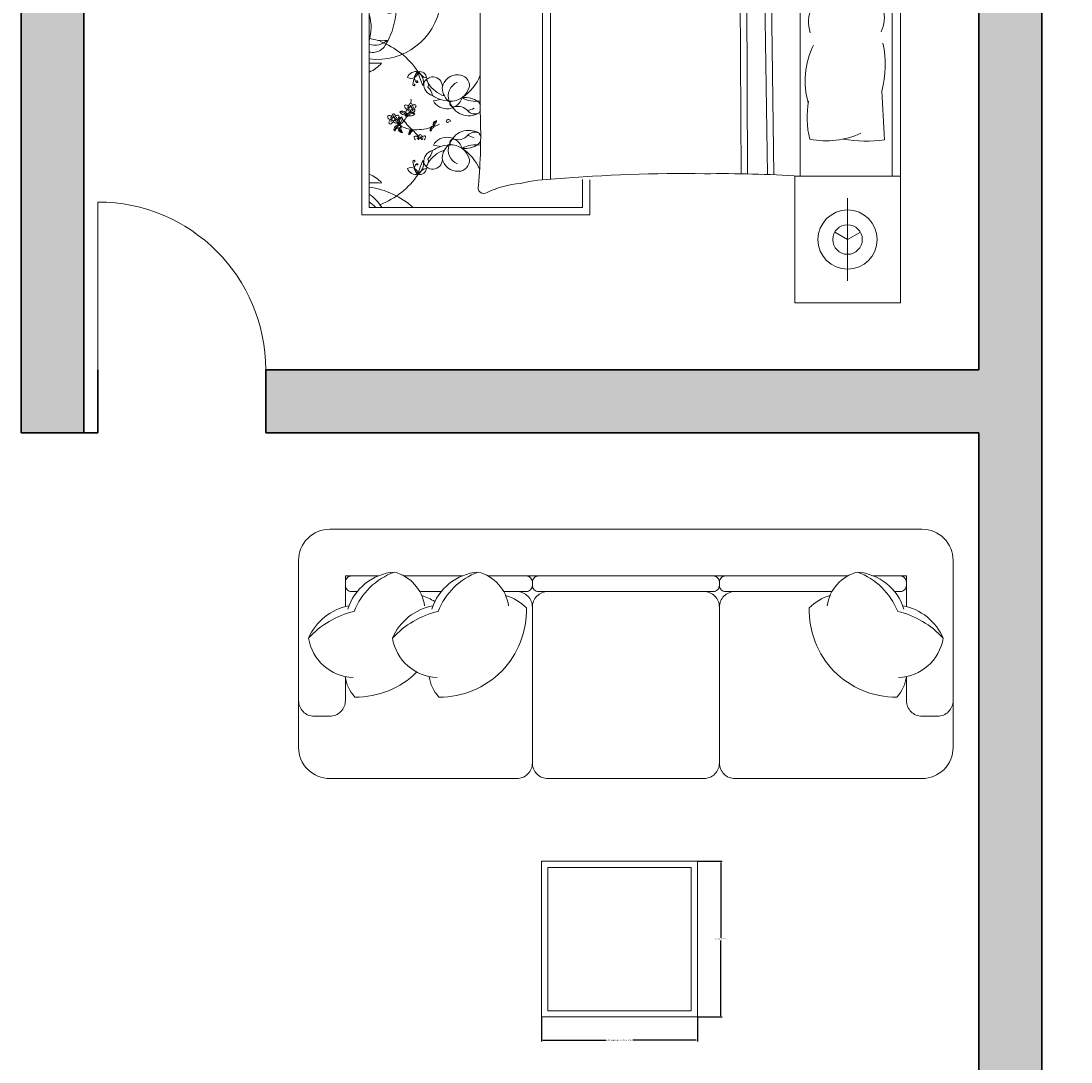
# Model space of a CAD drawing. Units: inches. Extents: x 37 to 706, y -568 to 110.
# Tile 19 of 24: x 212 to 362, y -233 to -84. Entities that reach past the tile are written whole.
import ezdxf

# ---------------------------------------------------------------- set-up
doc = ezdxf.new("R2010")
doc.units = ezdxf.units.IN
doc.header["$MEASUREMENT"] = 0
for name, color, linetype, lineweight in [('A-ANNO-DIMS', 2, 'Continuous', 18), ('A-DOOR', 4, 'Continuous', 18), ('A-FURN', 8, 'Continuous', 13), ('A-WALL', 7, 'Continuous', 35), ('A-WALL-PATT', 252, 'Continuous', 13)]:
    doc.layers.add(name, color=color, linetype=linetype, lineweight=lineweight)
doc.styles.get("Standard").update_dxf_attribs({"font": 'arial.ttf'})
doc.dimstyles.get("Standard").update_dxf_attribs({"dimtxt": 0.18, "dimasz": 0.18, "dimexe": 0.18, "dimexo": 0.0625, "dimgap": 0.09, "dimtad": 0, "dimtih": 1, "dimtoh": 1, "dimdec": 0, "dimzin": 0, "dimdsep": 46, "dimlunit": 3, "dimtxsty": 'Standard', "dimcen": 0.09, "dimadec": 0, "dimazin": 0, "dimtfac": 1, "dimtdec": 0, "dimtofl": 0, "dimtmove": 0, "dimatfit": 3, "dimfxl": 1, "dimtolj": 1, "dimtzin": 0, "dimarcsym": 0})

# ---------------------------------------------------------------- blocks, each defined once
blk = doc.blocks.new('BED-DOUBLE-WITH-NIGHTSTANDS')
for p, q in [((77.02, 90.57), (77.02, 0)), ((69.47, 75.59), (69.47, 87.43)), ((63.56, 81.51), (75.39, 81.51)), ((0, 78.61), (32.62, 78.61)), ((0, 12.59), (0, 78.61)), ((32.62, 78.61), (32.62, 73.49)), ((1.05, 77.56), (1.05, 13.64)), ((31.58, 77.56), (1.05, 77.56)), ((31.58, 73.49), (31.58, 77.56)), ((25.85, 17.62), (25.85, 73.5)), ((26.98, 17.7), (26.98, 73.5)), ((50.48, 72.53), (51.22, 73.26)), ((50.85, 68.86), (50.48, 72.53)), ((51.22, 73.26), (55.07, 69.96)), ((77.02, 72.45), (52.16, 72.45)), ((62.71, 72.45), (62.71, 18.11)), ((75.86, 18.11), (75.86, 72.45)), ((55.07, 69.96), (57.63, 66.48)), ((10.23, 68.64), (11.25, 68.84)), ((50.48, 64.28), (50.85, 68.86)), ((57.63, 66.48), (60.02, 59.87)), ((16.95, 26.9), (16.95, 63.67)), ((49.93, 60.24), (50.48, 64.28)), ((10.23, 62.31), (11.25, 62.11)), ((48.83, 57.86), (49.93, 60.24)), ((60.02, 59.87), (62.71, 50)), ((48.1, 54.92), (48.83, 57.86)), ((50.48, 54.55), (48.1, 54.92)), ((55.8, 52.54), (50.48, 54.55)), ((54.24, 18.43), (54.09, 53.18)), ((55.17, 18.44), (55.03, 52.83)), ((62.71, 47.57), (55.8, 52.54)), ((58.02, 18.39), (57.55, 51.28)), ((58.95, 18.36), (58.49, 50.6)), ((10.23, 28.89), (11.25, 29.09)), ((10.23, 22.56), (11.25, 22.36)), ((31.58, 13.64), (31.58, 17.63)), ((32.62, 17.61), (32.62, 12.59)), ((1.05, 13.64), (31.58, 13.64)), ((69.47, 14.97), (69.47, 3.14)), ((32.62, 12.59), (0, 12.59))]:
    blk.add_line(p, q)
for points in [[(61.93, 72.45), (61.93, 90.57), (77.02, 90.57)], [(69.47, 81.51), (67.64, 80.45)], [(69.47, 81.51), (71.3, 80.45)], [(77.02, 18.11), (61.93, 18.11), (61.93, 0), (77.02, 0)], [(69.47, 9.06), (67.64, 10.11)], [(69.47, 9.06), (71.3, 10.11)]]:
    blk.add_lwpolyline(points)
for points in [[(42.92, 73.45, 0.001242), (25.74, 73.5, -0.127202), (17.18, 75.31)], [(74.76, 67.25, 0.074897), (68.85, 67.14, -0.472817)], [(68.52, 45.71, 0.14099), (74.55, 45.53, 0.235245)], [(68.52, 41.84, -0.14099), (74.55, 42.02, -0.235245)], [(74.76, 23.32, -0.074897), (68.85, 23.42, 0.472817)], [(27.69, 17.73, 0.056112), (22.71, 17.07, 0.095341), (17.91, 15.8)]]:
    blk.add_lwpolyline(points, format="xyb")
for centre, radius in [((69.47, 81.51), 4.23), ((69.47, 81.51), 2.11), ((4.52, 64.91), 0.231), ((6.95, 63.41), 0.231), ((6.95, 27.79), 0.231), ((4.52, 26.28), 0.231), ((69.47, 9.06), 4.23), ((69.47, 9.06), 2.11)]:
    blk.add_circle(centre, radius)
for centre, radius, start, end in [((-3.2, 82.51), 7.18, 306.3036, 316.4814), ((-2.13, 80.43), 5.76, 303.4617, 330.1116), ((-0.54, 86.37), 11.83, 277.745, 311.8856), ((-1.71, 66.13), 11.83, 34.3865, 68.5908), ((17.23, 74.48), 0.836, 93.98, 207.3412), ((-0.79, 77.21), 4.81, 292.5547, 318.9546), ((1.79, 90.38), 16.36, 267.4081, 273.6519), ((-77.32, 64.75), 94.28, 359.3433, 5.6887), ((7.77, 71.53), 1.31, 77.7115, 159.0387), ((7.06, 72.84), 0.988, 238.4633, 358.2869), ((10.3, 70.85), 2.99, 138.8402, 177.9352), ((8.5, 71.96), 0.967, 117.6827, 223.7762), ((8.28, 71.86), 0.98, 2.9516, 103.728), ((16.12, 74.61), 8.27, 192.5173, 207.1824), ((6.95, 71.3), 1.87, 345.4653, 54.2343), ((9.77, 73.87), 2.02, 211.3827, 255.2969), ((13.65, 70.21), 2.16, 84.9449, 172.8857), ((13.86, 70.84), 1.53, 354.4856, 91.0538), ((48.97, 156.3), 83.07, 265.8294, 271.553), ((83.29, 71.71), 34.18, 177.4519, 191.3392), ((7.46, 70.95), 0.147, 177.9352, 11.4834), ((7.53, 70.96), 0.0713, 11.4834, 127.9409), ((7.89, 71.38), 0.128, 223.7762, 159.7183), ((10.16, 70.71), 1.36, 350.264, 160.8688), ((10.57, 71.04), 1.7, 175.969, 254.3045), ((8.69, 70.99), 0.833, 333.9755, 53.2681), ((8.31, 69.21), 1.81, 6.1662, 51.5825), ((13.15, 73.4), 4.28, 211.2614, 251.7045), ((14.47, 69.36), 2.1, 111.5819, 201.4221), ((12.73, 71.31), 2.72, 265.2933, 346.921), ((10.57, 74.83), 6.85, 303.6671, 333.2997), ((12.81, 73.44), 4.86, 236.2883, 266.5076), ((12.18, 69.76), 2.25, 209.9085, 343.1337), ((14.13, 70.59), 2.63, 182.3591, 234.0401), ((16.28, 72.32), 3.75, 238.8218, 279.1554), ((14.65, 65.65), 3.49, 55.785, 94.7304), ((7.66, 67.53), 0.177, 142.4737, 265.053), ((7.89, 67.56), 0.381, 127.7621, 169.0403), ((7.69, 67.89), 0.536, 265.053, 338.3618), ((8.4, 67.15), 0.7, 113.4276, 137.6104), ((8.32, 67.88), 0.231, 183.2768, 356.7232), ((8.49, 67.46), 0.377, 139.7889, 227.6792), ((7.6, 67.46), 0.755, 353.0852, 15.7171), ((8.1, 67.37), 0.477, 350.3487, 43.6538), ((8.98, 67.87), 0.555, 198.7263, 262.5032), ((8.54, 67.61), 0.22, 1.1081, 91.8675), ((8.68, 67.56), 0.385, 11.5637, 52.6358), ((8.95, 67.49), 0.178, 255.2356, 54.9248), ((13.13, 68.34), 0.562, 167.3041, 285.1471), ((14.65, 65.65), 3.49, 122.7011, 126.3445), ((15.31, 69.41), 2.89, 199.2822, 299.1751), ((13.76, 66), 1.86, 41.5653, 105.1471), ((14.78, 69.85), 2.6, 277.436, 299.9149), ((15.95, 67.67), 1.09, 30.0293, 52.325), ((4.85, 66.4), 0.258, 124.3538, 214.3923), ((5.23, 66.36), 0.6, 190.3057, 287.1958), ((5.41, 66.58), 0.697, 176.9701, 248.2913), ((10.38, 70.25), 6.74, 212.6784, 216.3746), ((5.17, 66.41), 0.267, 216.3746, 291.7548), ((5.81, 66.23), 0.6, 122.8155, 187.3992), ((5.34, 65.98), 0.201, 289.3605, 111.7548), ((5.49, 65.98), 0.201, 221.8703, 44.2646), ((6.07, 66.15), 0.697, 109.4799, 177.6828), ((5.7, 66.59), 0.258, 56.8636, 146.9021), ((5.83, 66.31), 0.267, 148.8844, 224.2646), ((11.37, 62.96), 6.74, 145.1882, 148.8844), ((7.53, 62.67), 3.76, 94.756, 119.2041), ((15.54, 57.26), 12.37, 132.2412, 142.1744), ((9.29, 67.11), 2.55, 178.3264, 187.1302), ((6.53, 66.75), 0.476, 11.3256, 64.4621), ((8.15, 67.44), 1.43, 190.2588, 210.656), ((7.19, 66.85), 0.435, 188.3432, 274.2869), ((7.57, 67.09), 0.759, 210.656, 242.6341), ((8.14, 67.75), 1.46, 218.2101, 226.3071), ((7.07, 66.52), 0.185, 325.7657, 67.4417), ((1.34, 72.69), 8.6, 313.1541, 322.0459), ((7.72, 58.94), 7.5, 73.5842, 93.8277), ((8.37, 67.33), 0.199, 227.6792, 350.3487), ((12.34, 66.57), 2.55, 178.3264, 187.1302), ((9.58, 66.21), 0.476, 11.3256, 64.4621), ((11.19, 66.9), 1.43, 190.2588, 210.656), ((10.23, 66.31), 0.435, 188.3432, 274.2869), ((10.61, 66.55), 0.759, 210.656, 242.6341), ((11.19, 67.21), 1.46, 218.2101, 226.3071), ((10.11, 65.98), 0.185, 325.7657, 67.4417), ((16.16, 68.13), 1.36, 221.5653, 293.8354), ((15.95, 67.67), 1.09, 314.4517, 333.558), ((75.82, 64.02), 12.14, 165.1039, 191.0369), ((66.47, 55.71), 11.67, 65.1316, 101.7583), ((936.66, 17.33), 863.34, 176.68521, 177.14978), ((3.86, 64.56), 0.177, 142.4737, 265.053), ((4.09, 64.6), 0.381, 61.2196, 169.0403), ((3.89, 64.92), 0.536, 265.053, 338.3618), ((4.34, 65.38), 0.455, 157.4086, 261.4386), ((4.09, 65.4), 0.229, 58.0499, 135.6268), ((4.6, 64.19), 0.7, 113.4276, 137.6104), ((4.32, 65.26), 0.153, 172.906, 277.132), ((3.82, 64.98), 0.727, 14.7558, 58.0499), ((4.69, 64.5), 0.377, 139.7889, 227.6792), ((4.84, 65.17), 0.315, 36.1046, 181.4281), ((3.8, 64.5), 0.755, 353.0852, 15.7171), ((4.29, 64.41), 0.477, 350.3487, 43.6538), ((5.18, 64.9), 0.555, 198.7263, 262.5032), ((4.66, 65.42), 0.317, 270.0645, 331.1507), ((4.93, 65.34), 0.363, 221.8413, 265.7877), ((4.74, 64.65), 0.22, 1.1081, 91.8675), ((4.92, 65.2), 0.226, 263.7526, 41.7054), ((4.88, 64.6), 0.385, 11.5637, 86.365), ((7.53, 62.67), 3.76, 124.0033, 132.4917), ((5.15, 64.53), 0.178, 255.2356, 54.9248), ((3.66, 62.2), 4.02, 63.7819, 68.2913), ((5.81, 65.29), 0.639, 128.3208, 208.8162), ((5.92, 65.34), 0.764, 207.7043, 254.3516), ((6.41, 65.39), 1.05, 157.2305, 229.0635), ((6.05, 65.74), 0.619, 174.4544, 220.6188), ((5.43, 64.9), 1.05, 270.278, 342.111), ((2.53, 62.29), 4.51, 30.544, 49.818), ((5.02, 64.86), 0.744, 340.0041, 40.6188), ((5.92, 64.93), 0.619, 278.7227, 324.8872), ((7.06, 64.61), 0.639, 182.8499, 266.1226), ((6.81, 65.06), 0.619, 231.7607, 277.9252), ((7.29, 65.17), 1.05, 214.5369, 286.3699), ((10.63, 65.65), 0.435, 147.5332, 233.4768), ((11.02, 65.87), 0.759, 179.1859, 211.164), ((10.28, 65.7), 0.185, 354.3784, 96.0543), ((7.72, 58.94), 7.5, 63.0032, 69.8941), ((11.6, 66.22), 1.43, 211.164, 231.5612), ((11.85, 67.38), 2.55, 234.6898, 243.4936), ((11.87, 66.07), 1.46, 195.5129, 203.6099), ((10.23, 65.12), 0.476, 357.3579, 50.4944), ((12.28, 65.21), 0.175, 12.7051, 190.4384), ((12.38, 65.23), 0.284, 190.4384, 10.4136), ((42.55, 63.54), 7.37, 336.2616, 11.3392), ((4.57, 64.37), 0.199, 227.6792, 350.3487), ((6.13, 63.58), 0.744, 98.7227, 159.3375), ((5.75, 64.54), 0.764, 244.9899, 291.6373), ((5.81, 64.43), 0.639, 290.5253, 358.5375), ((6.29, 63.06), 0.177, 142.4737, 265.053), ((6.52, 63.09), 0.381, 61.2196, 169.0403), ((6.32, 63.41), 0.536, 265.053, 338.3618), ((6.77, 63.88), 0.455, 157.4086, 261.4386), ((6.52, 63.89), 0.229, 58.0499, 135.6268), ((7.03, 62.68), 0.7, 113.4276, 137.6104), ((6.76, 63.75), 0.153, 172.906, 277.132), ((6.25, 63.47), 0.727, 14.7558, 58.0499), ((2.53, 62.29), 4.51, 23.0501, 23.8477), ((7.12, 62.99), 0.377, 139.7889, 227.6792), ((7, 63.71), 0.744, 37.3105, 97.9252), ((7.27, 63.66), 0.315, 36.1046, 181.4281), ((6.23, 62.99), 0.755, 353.0852, 15.7171), ((7.08, 64.73), 0.764, 265.0106, 311.658), ((6.72, 62.9), 0.477, 350.3487, 43.6538), ((7.61, 63.4), 0.555, 198.7263, 262.5032), ((7.09, 63.91), 0.317, 270.0645, 331.1507), ((7.36, 63.83), 0.363, 221.8413, 265.7877), ((7.17, 63.14), 0.22, 1.1081, 91.8675), ((7.36, 63.7), 0.226, 263.7526, 41.7054), ((7.31, 63.09), 0.385, 11.5637, 86.365), ((7.58, 63.02), 0.178, 255.2356, 54.9248), ((12.18, 61.19), 2.25, 16.8663, 150.0915), ((13.13, 62.61), 0.562, 74.8529, 192.6959), ((15.31, 61.54), 2.89, 60.8249, 160.7178), ((13.76, 64.95), 1.86, 254.8529, 318.4347), ((14.78, 61.1), 2.6, 60.0851, 82.564), ((16.16, 62.82), 1.36, 66.1646, 138.4347), ((15.95, 63.28), 1.09, 23.229, 45.5483), ((7, 62.86), 0.199, 227.6792, 350.3487), ((2.53, 62.29), 4.51, 357.1071, 4.7585), ((13.15, 57.54), 4.28, 108.2955, 148.7386), ((12.81, 57.5), 4.86, 93.4924, 123.7117), ((14.13, 60.36), 2.63, 125.9599, 177.6409), ((14.47, 61.59), 2.1, 158.5779, 248.4181), ((12.73, 59.64), 2.72, 13.079, 94.7067), ((14.65, 65.3), 3.49, 233.6555, 237.2989), ((16.28, 58.63), 3.75, 79.7133, 121.1782), ((14.65, 65.3), 3.49, 265.2696, 304.215), ((10.57, 56.11), 6.85, 21.4941, 56.3329), ((15.95, 63.28), 1.09, 307.675, 336.7144), ((84.45, 57.63), 21.05, 168.0397, 199.2615), ((7.46, 60), 0.147, 348.5166, 182.0648), ((6.95, 59.65), 1.87, 305.7657, 14.5347), ((16.12, 56.34), 8.27, 152.8176, 167.4827), ((10.57, 59.91), 1.7, 105.6955, 184.031), ((10.16, 60.24), 1.36, 199.1312, 9.736), ((8.69, 59.96), 0.833, 306.7319, 26.0245), ((8.31, 61.74), 1.81, 308.4175, 353.8338), ((13.65, 60.74), 2.16, 187.1143, 275.0551), ((13.86, 60.11), 1.53, 268.9462, 5.5144), ((82.33, 48.63), 35.12, 160.1194, 169.3383), ((41.99, 54.84), 32.85, 352.2196, 9.497), ((7.06, 58.1), 0.988, 1.7131, 121.5367), ((7.77, 59.41), 1.31, 200.9613, 282.2885), ((10.3, 60.1), 2.99, 182.0648, 221.1598), ((7.53, 59.98), 0.0713, 232.0591, 348.5166), ((8.5, 58.99), 0.967, 136.2238, 242.3173), ((7.94, 59.56), 0.0771, 200.2667, 136.2271), ((8.28, 59.09), 0.98, 256.272, 357.0484), ((9.77, 57.08), 2.02, 104.7031, 148.6173), ((-0.79, 53.74), 4.81, 41.0454, 67.4453), ((-1.71, 64.81), 11.83, 291.4092, 325.6135), ((1.79, 40.57), 16.36, 86.3481, 92.5919), ((-0.54, 44.58), 11.83, 4.4623, 82.255), ((-2.13, 50.51), 5.76, 1.272, 56.5383), ((-3.2, 48.44), 7.18, 17.8504, 53.6964), ((48.03, 55.13), 0.219, 178.8623, 289.7536), ((-5.22, 44.66), 10.68, 34.0123, 54.053), ((79.85, 49.11), 15.97, 169.8617, 193.6238), ((58.59, 47.9), 16.14, 351.5249, 13.96), ((-5.17, 48.79), 6.5, 343.5431, 17.0202), ((-6.88, 45.48), 11.83, 4.4623, 27.4146), ((-8.52, 46.22), 9.62, 4.3787, 5.6357), ((-15.11, 41.15), 17.18, 19.7217, 19.9028), ((4.03, 45.43), 1.31, 47.7873, 129.1145), ((4.07, 46.92), 0.988, 208.5391, 328.3627), ((3.47, 45.08), 0.147, 148.011, 341.5592), ((5.88, 43.58), 2.99, 108.9159, 148.011), ((3.54, 45.06), 0.0713, 341.5592, 98.0167), ((4.87, 45.44), 0.967, 87.7585, 193.852), ((4.06, 45.24), 0.128, 193.852, 129.9245), ((12.81, 43.93), 8.27, 162.593, 177.2582), ((3.21, 45.64), 1.87, 315.5411, 24.3101), ((6.93, 46.46), 2.02, 181.4585, 225.3727), ((4.64, 45.46), 0.98, 333.0274, 73.8037), ((10.37, 44.53), 1.31, 47.7873, 129.1145), ((10.41, 46.02), 0.988, 208.5391, 328.3627), ((12.22, 42.67), 2.99, 108.9159, 148.011), ((11.21, 44.53), 0.967, 87.7585, 193.852), ((9.54, 44.73), 1.87, 315.5411, 24.3101), ((19.14, 43.02), 8.27, 162.593, 177.2582), ((10.97, 44.56), 0.98, 333.0274, 73.8037), ((13.27, 45.55), 2.02, 181.4585, 225.3727), ((65.49, 56.38), 11.1, 264.0129, 285.8293), ((12.81, 44.25), 8.27, 182.7418, 197.407), ((3.21, 42.54), 1.87, 335.6899, 44.4589), ((9.8, 44.18), 0.147, 148.011, 341.5592), ((9.8, 44), 0.147, 18.4408, 211.989), ((12.22, 45.51), 2.99, 211.989, 251.0841), ((9.88, 44.15), 0.0713, 341.5592, 98.0167), ((9.88, 44.03), 0.0713, 261.9833, 18.4408), ((11.21, 43.65), 0.967, 166.148, 272.2415), ((10.39, 44.33), 0.128, 193.852, 129.9245), ((10.44, 43.86), 0.0771, 230.1909, 166.0209), ((9.54, 43.45), 1.87, 335.6899, 44.4589), ((19.14, 45.16), 8.27, 182.7418, 197.407), ((10.97, 43.62), 0.98, 286.1963, 26.9726), ((13.27, 42.63), 2.02, 134.6273, 178.5415), ((2.19, 43.98), 9.15, 262.8636, 351.8197), ((4.07, 41.26), 0.988, 31.6373, 151.4609), ((3.47, 43.1), 0.147, 18.4408, 211.989), ((5.88, 44.6), 2.99, 211.989, 251.0841), ((3.54, 43.12), 0.0713, 261.9833, 18.4408), ((4.87, 42.74), 0.967, 166.148, 272.2415), ((4.11, 42.95), 0.0771, 230.1909, 166.0209), ((6.93, 41.72), 2.02, 134.6273, 178.5415), ((4.64, 42.72), 0.98, 286.1963, 26.9726), ((10.41, 42.16), 0.988, 31.6373, 151.4609), ((10.37, 43.65), 1.31, 230.8855, 312.2127), ((68.68, 40.17), 4.8, 155.0183, 198.5407), ((65.49, 31.16), 11.1, 74.1707, 95.9871), ((-5.17, 39.39), 6.5, 342.9798, 16.4569), ((-8.52, 41.96), 9.62, 354.3643, 355.6213), ((-15.11, 47.03), 17.18, 340.0972, 340.2783), ((4.03, 42.75), 1.31, 230.8855, 312.2127), ((-6.88, 42.69), 11.83, 332.5854, 355.5377), ((70.25, 40.78), 4.48, 333.3437, 16.1026), ((3.02, 42.8), 5.3, 248.117, 276.6195), ((1.55, 37.94), 2.12, 256.3898, 349.0739), ((1.84, 39.54), 2.68, 252.8609, 311.9049), ((-1.71, 26.39), 11.83, 34.3865, 68.5908), ((74.93, 31.78), 11.53, 153.8761, 196.1746), ((58.92, 34.06), 15.92, 346.3427, 11.1841), ((1.79, 50.63), 16.36, 267.4081, 273.6519), ((-0.79, 37.46), 4.81, 292.5547, 318.9546), ((7.77, 31.78), 1.31, 77.7115, 159.0387), ((7.06, 33.09), 0.988, 238.4633, 358.2869), ((10.3, 31.1), 2.99, 138.8402, 177.9352), ((8.5, 32.21), 0.967, 117.6827, 223.7762), ((8.28, 32.11), 0.98, 2.9516, 103.728), ((9.77, 34.12), 2.02, 211.3827, 255.2969), ((6.95, 31.55), 1.87, 345.4653, 54.2343), ((16.12, 34.86), 8.27, 192.5173, 207.1824), ((7.89, 31.63), 0.128, 223.7762, 159.7183), ((10.16, 30.96), 1.36, 350.264, 160.8688), ((8.69, 31.24), 0.833, 333.9755, 53.2681), ((13.65, 30.46), 2.16, 84.9449, 172.8857), ((14.47, 29.61), 2.1, 111.5819, 201.4221), ((13.86, 31.09), 1.53, 354.4856, 91.0538), ((10.57, 35.08), 6.85, 303.6671, 338.5059), ((7.46, 31.2), 0.147, 177.9352, 11.4834), ((7.53, 31.21), 0.0713, 11.4834, 127.9409), ((10.57, 31.29), 1.7, 175.969, 254.3045), ((8.31, 29.46), 1.81, 6.1662, 51.5825), ((13.15, 33.66), 4.28, 211.2614, 251.7045), ((14.13, 30.84), 2.63, 182.3591, 234.0401), ((12.73, 31.56), 2.72, 265.2933, 346.921), ((936.66, 73.23), 863.34, 182.85022, 183.31479), ((7, 28.34), 0.199, 9.6513, 132.3208), ((2.53, 28.91), 4.51, 355.2415, 2.8929), ((12.81, 33.7), 4.86, 236.2883, 266.5076), ((12.18, 30.01), 2.25, 209.9085, 343.1337), ((13.13, 28.59), 0.562, 167.3041, 285.1471), ((14.65, 25.9), 3.49, 122.7011, 126.3445), ((15.31, 29.66), 2.89, 199.2822, 299.1751), ((16.28, 32.57), 3.75, 238.8218, 280.2867), ((14.65, 25.9), 3.49, 55.785, 94.7304), ((15.95, 27.92), 1.09, 23.2856, 52.325), ((75.82, 26.55), 12.14, 168.9631, 194.8961), ((4.57, 26.83), 0.199, 9.6513, 132.3208), ((5.75, 26.66), 0.764, 68.3627, 115.0101), ((5.43, 26.3), 1.05, 17.889, 89.722), ((6.13, 27.61), 0.744, 200.6625, 261.2773), ((5.81, 26.77), 0.639, 1.4625, 69.4747), ((6.29, 28.14), 0.177, 94.947, 217.5263), ((6.52, 28.11), 0.381, 190.9597, 298.7804), ((6.32, 27.78), 0.536, 21.6382, 94.947), ((6.77, 27.32), 0.455, 98.5614, 202.5914), ((6.52, 27.31), 0.229, 224.3732, 301.9501), ((7.06, 26.59), 0.639, 93.8774, 177.1501), ((7.29, 26.03), 1.05, 73.6301, 145.4631), ((7.03, 28.52), 0.7, 222.3896, 246.5724), ((6.76, 27.45), 0.153, 82.868, 187.094), ((6.25, 27.73), 0.727, 301.9501, 345.2442), ((2.53, 28.91), 4.51, 336.1523, 336.9499), ((7.12, 28.21), 0.377, 132.3208, 220.2111), ((7, 27.49), 0.744, 262.0748, 322.6895), ((6.23, 28.2), 0.755, 344.2829, 6.9148), ((7.27, 27.54), 0.315, 178.5719, 323.8954), ((7.08, 26.46), 0.764, 48.342, 94.9894), ((6.72, 28.3), 0.477, 316.3462, 9.6513), ((7.61, 27.8), 0.555, 97.4968, 161.2737), ((7.36, 27.37), 0.363, 94.2123, 138.1587), ((7.09, 27.29), 0.317, 28.8493, 89.9355), ((7.17, 28.06), 0.22, 268.1325, 358.8919), ((7.31, 28.11), 0.385, 273.635, 348.4363), ((7.36, 27.5), 0.226, 318.2946, 96.2474), ((7.58, 28.18), 0.178, 305.0752, 104.7644), ((13.76, 26.25), 1.86, 41.5653, 105.1471), ((14.78, 30.1), 2.6, 277.436, 299.9149), ((16.16, 28.38), 1.36, 221.5653, 293.8354), ((15.95, 27.92), 1.09, 314.4517, 336.7144), ((3.86, 26.63), 0.177, 94.947, 217.5263), ((4.09, 26.6), 0.381, 190.9597, 298.7804), ((3.89, 26.28), 0.536, 21.6382, 94.947), ((4.34, 25.81), 0.455, 98.5614, 202.5914), ((4.09, 25.8), 0.229, 224.3732, 301.9501), ((4.6, 27.01), 0.7, 222.3896, 246.5724), ((4.32, 25.94), 0.153, 82.868, 187.094), ((3.82, 26.22), 0.727, 301.9501, 345.2442), ((4.69, 26.7), 0.377, 132.3208, 220.2111), ((4.84, 26.03), 0.315, 178.5719, 323.8954), ((3.8, 26.7), 0.755, 344.2829, 6.9148), ((4.29, 26.79), 0.477, 316.3462, 9.6513), ((5.18, 26.29), 0.555, 97.4968, 161.2737), ((4.93, 25.86), 0.363, 94.2123, 138.1587), ((4.66, 25.78), 0.317, 28.8493, 89.9355), ((4.74, 26.55), 0.22, 268.1325, 358.8919), ((4.88, 26.6), 0.385, 273.635, 348.4363), ((4.92, 25.99), 0.226, 318.2946, 96.2474), ((7.53, 28.53), 3.76, 227.5083, 235.9967), ((5.15, 26.67), 0.178, 305.0752, 104.7644), ((5.81, 25.91), 0.639, 151.1838, 231.6792), ((5.92, 25.86), 0.764, 105.6484, 152.2957), ((6.41, 25.8), 1.05, 130.9365, 202.7695), ((6.05, 25.46), 0.619, 139.3812, 185.5456), ((2.53, 28.91), 4.51, 310.182, 329.456), ((5.02, 26.34), 0.744, 319.3812, 19.9959), ((15.54, 33.94), 12.37, 217.8256, 227.7588), ((5.92, 26.27), 0.619, 35.1128, 81.2773), ((6.81, 26.14), 0.619, 82.0748, 128.2393), ((10.63, 25.55), 0.435, 126.5232, 212.4668), ((11.02, 25.33), 0.759, 148.836, 180.8141), ((7.72, 32.26), 7.5, 290.1059, 296.9968), ((11.6, 24.98), 1.43, 128.4388, 148.836), ((11.85, 23.82), 2.55, 116.5064, 125.3102), ((11.87, 25.13), 1.46, 156.3901, 164.4871), ((10.23, 26.08), 0.476, 309.5056, 2.6421), ((12.28, 25.98), 0.175, 169.5616, 347.2949), ((12.38, 25.96), 0.284, 349.5864, 169.5616), ((-71.13, 24.12), 88.13, 355.2402, 1.8035), ((4.85, 24.8), 0.258, 145.6077, 235.6462), ((5.23, 24.83), 0.6, 72.8042, 169.6943), ((5.41, 24.62), 0.697, 111.7087, 183.0299), ((10.38, 20.95), 6.74, 143.6254, 147.3216), ((5.17, 24.78), 0.267, 68.2452, 143.6254), ((3.66, 29), 4.02, 291.7087, 296.2181), ((5.81, 24.97), 0.6, 172.6008, 237.1845), ((5.34, 25.22), 0.201, 248.2452, 70.6395), ((5.49, 25.22), 0.201, 315.7354, 138.1297), ((6.07, 25.05), 0.697, 182.3172, 250.5201), ((5.7, 24.61), 0.258, 213.0979, 303.1364), ((5.83, 24.89), 0.267, 135.7354, 211.1156), ((11.37, 28.24), 6.74, 211.1156, 214.8118), ((7.53, 28.53), 3.76, 240.7959, 265.244), ((8.15, 23.76), 1.43, 149.344, 169.7412), ((9.29, 24.09), 2.55, 172.8698, 181.6736), ((6.53, 24.45), 0.476, 295.5379, 348.6744), ((7.19, 24.34), 0.435, 85.7131, 171.6568), ((7.57, 24.1), 0.759, 117.3659, 149.344), ((8.14, 23.45), 1.46, 133.6929, 141.7899), ((7.07, 24.67), 0.185, 292.5583, 34.2343), ((7.72, 32.26), 7.5, 266.1723, 286.4158), ((1.34, 18.5), 8.6, 37.9541, 46.8459), ((8.37, 23.87), 0.199, 9.6513, 132.3208), ((11.19, 24.3), 1.43, 149.344, 169.7412), ((12.34, 24.63), 2.55, 172.8698, 181.6736), ((9.58, 24.98), 0.476, 295.5379, 348.6744), ((10.23, 24.88), 0.435, 85.7131, 171.6568), ((10.61, 24.64), 0.759, 117.3659, 149.344), ((11.19, 23.99), 1.46, 133.6929, 141.7899), ((10.11, 25.21), 0.185, 292.5583, 34.2343), ((10.28, 25.5), 0.185, 263.9457, 5.6216), ((15.31, 21.79), 2.89, 60.8249, 160.7178), ((16.16, 23.07), 1.36, 66.1646, 138.4347), ((15.95, 23.53), 1.09, 16.6343, 45.5483), ((66.47, 34.85), 11.67, 258.2417, 294.8684), ((7.66, 23.67), 0.177, 94.947, 217.5263), ((7.89, 23.64), 0.381, 190.9597, 232.2379), ((7.69, 23.31), 0.536, 21.6382, 94.947), ((8.4, 24.05), 0.7, 222.3896, 246.5724), ((8.32, 23.32), 0.231, 3.2768, 176.7232), ((8.49, 23.74), 0.377, 132.3208, 220.2111), ((7.6, 23.73), 0.755, 344.2829, 6.9148), ((8.1, 23.82), 0.477, 316.3462, 9.6513), ((8.98, 23.33), 0.555, 97.4968, 161.2737), ((8.54, 23.59), 0.22, 268.1325, 358.8919), ((8.95, 23.71), 0.178, 305.0752, 104.7644), ((8.68, 23.64), 0.385, 307.3642, 348.4363), ((12.81, 17.75), 4.86, 93.4924, 123.7117), ((12.18, 21.44), 2.25, 16.8663, 150.0915), ((14.13, 20.61), 2.63, 125.9599, 177.6409), ((14.47, 21.84), 2.1, 158.5779, 248.4181), ((12.73, 19.89), 2.72, 13.079, 94.7067), ((13.13, 22.86), 0.562, 74.8529, 192.6959), ((14.65, 25.55), 3.49, 233.6555, 237.2989), ((13.76, 25.2), 1.86, 254.8529, 318.4347), ((16.28, 18.88), 3.75, 79.249, 121.1782), ((14.65, 25.55), 3.49, 265.2696, 304.215), ((14.78, 21.35), 2.6, 60.0851, 82.564), ((15.95, 23.53), 1.09, 307.675, 342.5814), ((10.57, 20.16), 1.7, 105.6955, 184.031), ((8.31, 21.99), 1.81, 308.4175, 353.8338), ((13.15, 17.79), 4.28, 108.2955, 148.7386), ((10.57, 16.37), 6.85, 23.6453, 56.3329), ((7.46, 20.25), 0.147, 348.5166, 182.0648), ((10.3, 20.35), 2.99, 182.0648, 221.1598), ((7.53, 20.24), 0.0713, 232.0591, 348.5166), ((8.5, 19.24), 0.967, 136.2238, 242.3173), ((7.94, 19.81), 0.0771, 200.2667, 136.2271), ((16.12, 16.59), 8.27, 152.8176, 167.4827), ((6.95, 19.9), 1.87, 305.7657, 14.5347), ((10.16, 20.49), 1.36, 199.1312, 9.736), ((8.69, 20.21), 0.833, 306.7319, 26.0245), ((13.65, 20.99), 2.16, 187.1143, 275.0551), ((13.86, 20.36), 1.53, 268.9462, 5.5144), ((-0.79, 13.99), 4.81, 41.0454, 67.4453), ((-1.71, 25.06), 11.83, 291.4092, 325.6135), ((7.06, 18.36), 0.988, 1.7131, 121.5367), ((7.77, 19.67), 1.31, 200.9613, 282.2885), ((9.77, 17.33), 2.02, 104.7031, 148.6173), ((8.28, 19.34), 0.98, 256.272, 357.0484), ((45.72, -193.78), 212.28, 89.1145, 94.8735), ((51.64, -144.24), 162.73, 86.1, 90.9282), ((1.79, 0.82), 16.36, 86.3481, 92.5919), ((-0.54, 4.83), 11.83, 48.1144, 82.255), ((17.45, 16.48), 0.826, 156.5219, 303.8264), ((-2.13, 10.76), 5.76, 29.8884, 56.5383), ((-3.2, 8.69), 7.18, 43.5186, 53.6964)]:
    blk.add_arc(centre, radius, start, end)
blk = doc.blocks.new('COFFEE-TABLE-SQUARE')
at = {"ltscale": 0.03}
blk.add_lwpolyline([(22.29, 0), (0, 0), (0, 22.29), (22.29, 22.29)], close=True, dxfattribs=at)
blk.add_lwpolyline([(0.89, 0.89), (21.4, 0.89), (21.4, 21.4), (0.89, 21.4)], close=True)
blk = doc.blocks.new('DOOR-SWING-24')
blk.add_line((0, 0), (0, 24))
blk.add_arc((0, 0), 24, 0, 90)
blk = doc.blocks.new('*D35')
at = {"layer": 'A-ANNO-DIMS', "color": 0, "lineweight": -2, "transparency": 16777216}
for p, q in [((286.42, -226.33), (286.42, -229.79)), ((308.71, -226.33), (308.71, -229.79)), ((286.6, -229.61), (295.67, -229.61)), ((308.53, -229.61), (299.46, -229.61))]:
    blk.add_line(p, q, dxfattribs=at)
at = {"layer": 'A-ANNO-DIMS', "color": 0, "transparency": 16777216}
for points in [[(286.6, -229.58), (286.6, -229.64), (286.42, -229.61)], [(308.53, -229.58), (308.53, -229.64), (308.71, -229.61)]]:
    blk.add_solid(points, dxfattribs=at)
at = {"layer": 'Defpoints', "color": 0, "transparency": 16777216}
for p in [(286.42, -226.27), (308.71, -226.27), (308.71, -229.61)]:
    blk.add_point(p, dxfattribs=at)
at = {"layer": 'A-ANNO-DIMS', "color": 0, "transparency": 16777216, "insert": (297.56, -229.61), "char_height": 0.18, "attachment_point": 5}
blk.add_mtext('\\A1;COFFEE TABLE 1\'-10 1/2" TYP.', dxfattribs=at)
blk = doc.blocks.new('*D36')
at = {"layer": 'A-ANNO-DIMS', "color": 0, "lineweight": -2, "transparency": 16777216}
for p, q in [((308.77, -203.98), (312.23, -203.98)), ((312.05, -204.16), (312.05, -214.94)), ((312.05, -226.09), (312.05, -215.31)), ((308.77, -226.27), (312.23, -226.27))]:
    blk.add_line(p, q, dxfattribs=at)
at = {"layer": 'A-ANNO-DIMS', "color": 0, "transparency": 16777216}
for points in [[(312.02, -204.16), (312.08, -204.16), (312.05, -203.98)], [(312.02, -226.09), (312.08, -226.09), (312.05, -226.27)]]:
    blk.add_solid(points, dxfattribs=at)
at = {"layer": 'Defpoints', "color": 0, "transparency": 16777216}
for p in [(308.71, -203.98), (312.05, -203.98), (308.71, -226.27)]:
    blk.add_point(p, dxfattribs=at)
at = {"layer": 'A-ANNO-DIMS', "color": 0, "transparency": 16777216, "insert": (312.05, -215.12), "char_height": 0.18, "attachment_point": 5}
blk.add_mtext('\\A1;1\'-10 1/2" TYP.', dxfattribs=at)

msp = doc.modelspace()

# ---------------------------------------------------------------- hatches: boundary and pattern name
at = {"layer": 'A-WALL-PATT'}
h = msp.add_hatch(color=256, dxfattribs=at)
h.dxf.hatch_style = 1
h.paths.add_polyline_path([(220.96, -351.71), (211.96, -351.71), (211.96, -513.71), (254.96, -513.71), (254.96, -504.71), (220.96, -504.71)], flags=17)
h.paths.add_polyline_path([(220.96, -294.71), (211.96, -294.71), (211.96, -303.71), (220.96, -303.71)], flags=17)
h.paths.add_polyline_path([(175.96, -294.71), (155.87, -294.71), (155.87, -303.71), (155.96, -303.71), (175.96, -303.71)], flags=17)
h.paths.add_polyline_path([(220.96, -16.71), (211.96, -16.71), (211.96, -142.71), (220.96, -142.71)], flags=17)
h.paths.add_polyline_path([(357.96, 51.29), (78.96, 51.29), (78.96, -513.71), (87.96, -513.71), (87.96, -303.71), (95.87, -303.71), (95.87, -294.71), (87.96, -294.71), (87.96, -142.71), (187.96, -142.71), (187.96, -133.71), (87.96, -133.71), (87.96, -25.71), (106.96, -25.71), (106.96, -16.71), (87.96, -16.71), (87.96, 42.29), (348.96, 42.29), (348.96, 17.13), (348.96, -133.71), (246.96, -133.71), (246.96, -142.71), (348.96, -142.71), (348.96, -294.71), (251.96, -294.71), (251.96, -303.71), (348.96, -303.71), (348.96, -351.71), (260.96, -351.71), (260.96, -329.71), (251.96, -329.71), (251.96, -360.71), (327.45, -360.71), (348.96, -360.71), (348.96, -504.71), (314.96, -504.71), (314.96, -513.71), (357.96, -513.71)])
h.paths.add_polyline_path([(416.96, -303.71), (402.96, -303.71), (402.96, -151.71), (478.96, -151.71), (478.96, -142.71), (402.96, -142.71), (402.96, -22.71), (409.96, -22.71), (409.96, -13.71), (402.96, -13.71), (402.96, 42.29), (663.96, 42.29), (663.96, -303.71), (566.96, -303.71), (566.96, -312.71), (663.96, -312.71), (663.96, -360.71), (575.96, -360.71), (575.96, -338.71), (566.96, -338.71), (566.96, -360.71), (566.96, -369.71), (642.45, -369.71), (663.96, -369.71), (663.96, -513.71), (629.96, -513.71), (629.96, -522.71), (672.96, -522.71), (672.96, 51.29), (393.96, 51.29), (393.96, -522.71), (402.96, -522.71), (402.96, -312.71), (416.96, -312.71)])
h.paths.add_polyline_path([(490.96, -303.71), (476.96, -303.71), (476.96, -312.71), (490.96, -312.71)], flags=17)
h.paths.add_polyline_path([(535.96, -303.71), (526.96, -303.71), (526.96, -312.71), (535.96, -312.71)], flags=17)
h.paths.add_polyline_path([(535.96, -369.71), (526.96, -369.71), (526.96, -522.71), (569.96, -522.71), (569.96, -513.71), (535.96, -513.71)], flags=17)
h.paths.add_polyline_path([(511.96, -13.71), (502.96, -13.71), (502.96, -151.71), (511.96, -151.71)], flags=17)
h.paths.add_polyline_path([(651.54, -142.71), (651.54, -120.18), (642.54, -120.18), (642.54, -142.71), (550.54, -142.71), (550.54, -120.71), (541.54, -120.71), (541.54, -142.71), (537.96, -142.71), (537.96, -151.71), (651.54, -151.71)], flags=17)
h.paths.add_polyline_path([(651.54, -85.71), (541.54, -85.71), (541.54, -94.71), (651.54, -94.71)], flags=17)
h.paths.add_polyline_path([(476.96, -13.71), (469.96, -13.71), (469.96, -22.71), (476.96, -22.71)], flags=17)
h.paths.add_polyline_path([(185.96, -16.71), (166.96, -16.71), (166.96, -25.71), (185.96, -25.71)], flags=17)
h.paths.add_polyline_path([(168.91, -414.72), (214.62, -414.72), (214.62, -392.33), (168.91, -392.33)], flags=25)

# ---------------------------------------------------------------- linework, layer by layer
at = {"layer": 'A-FURN', "ltscale": 0.03}
msp.add_lwpolyline([(345.27, -187.71, -0.414214), (340.81, -192.17), (314.07, -192.17, -0.414214), (311.84, -189.94, -0.414214), (309.61, -192.17), (287.32, -192.17, -0.414214), (285.09, -189.94, -0.414214), (282.86, -192.17), (256.12, -192.17, -0.414214), (251.66, -187.71), (251.66, -160.97, -0.414214), (256.12, -156.51), (340.81, -156.51, -0.414214), (345.27, -160.97)], format="xyb", close=True, dxfattribs=at)
at = {"layer": 'A-FURN'}
for points in [[(253.08, -172.09, -0.14773), (259.59, -168.26, -0.213343), (265.34, -162.64, -0.178662)], [(263.03, -163.19), (258.35, -163.19), (258.35, -167.57, -0.414214)], [(260.05, -165.42), (259.24, -165.42, -0.414214), (258.35, -164.53), (258.35, -164.09, -0.414214), (259.24, -163.19)], [(258.69, -167.95, -0.306663), (265.34, -162.64, -0.30633), (269.68, -167.49, 0.872847)], [(259.24, -163.19), (263.03, -163.19, -0.414214)], [(265.08, -172.09, -0.14773), (271.6, -168.26, -0.213343), (277.35, -162.64, -0.178662)], [(266.74, -163.19), (275.04, -163.19, -0.414214)], [(270.7, -167.95, -0.306663), (277.35, -162.64, -0.30633), (281.69, -167.49, 0.872847)], [(278.75, -163.19), (284.2, -163.19, -0.414214), (285.09, -164.09), (285.09, -164.53, -0.414214), (284.2, -165.42), (280.99, -165.42, -0.414214)], [(330.19, -163.19), (312.73, -163.19, 0.414214), (311.84, -164.09), (311.84, -164.53, 0.414214), (312.73, -165.42), (327.94, -165.42, 0.414214)], [(338.24, -167.95, 0.306663), (331.59, -162.64, 0.30633), (327.25, -167.49, -0.872847)], [(343.85, -172.09, 0.14773), (337.34, -168.26, 0.213343), (331.59, -162.64, 0.178662)], [(337.69, -163.19), (333.9, -163.19, 0.414214)], [(336.88, -165.42), (337.69, -165.42, 0.414214), (338.59, -164.53), (338.59, -164.09, 0.414214), (337.69, -163.19)], [(272.05, -165.42), (268.99, -165.42, -0.414214)], [(271.13, -166.86, 0.071865), (269.27, -165.99, -7.115464)], [(270.35, -177.57, 0.165541), (271.73, -180.52, 0.425989), (284.24, -167.75, 0.121523), (281.27, -165.99, -7.115464)], [(282.86, -165.42, -0.414214), (285.09, -167.65), (285.09, -189.94, -0.414214)], [(287.32, -165.42, 0.414214), (285.09, -167.65)], [(309.61, -165.42, -0.414214), (311.84, -167.65)], [(314.07, -165.42, 0.414214), (311.84, -167.65), (311.84, -189.94, 0.414214)], [(338.59, -177.57, -0.165541), (337.21, -180.52, -0.425989), (324.69, -167.75, -0.121523), (327.66, -165.99, 7.115464)], [(259.46, -177.71, -0.356772), (253.08, -172.09, -0.249542), (258.86, -167.46, 9.61688)], [(271.47, -177.71, -0.356772), (265.08, -172.09, -0.249542), (270.87, -167.46, 9.61688)], [(337.47, -177.71, 0.356772), (343.85, -172.09, 0.249542), (338.07, -167.46, -9.61688)], [(258.34, -177.57, 0.165541), (259.72, -180.52, 0.200231), (268.57, -176.93, 0.121523)], [(258.35, -177.57), (258.35, -181.03, -0.414214), (256.12, -183.25), (253.89, -183.25, -0.414214), (251.66, -181.03)], [(345.27, -181.03, -0.414214), (343.04, -183.25), (340.81, -183.25, -0.414214), (338.59, -181.03), (338.59, -177.57)]]:
    msp.add_lwpolyline(points, format="xyb", dxfattribs=at)
for points in [[(275.04, -163.19), (266.74, -163.19)], [(330.19, -163.19), (278.75, -163.19)], [(338.59, -167.57), (338.59, -163.19), (333.9, -163.19)]]:
    msp.add_lwpolyline(points, dxfattribs=at)
msp.add_lwpolyline([(285.98, -163.19), (310.95, -163.19, -0.414214), (311.84, -164.09), (311.84, -164.53, -0.414214), (310.95, -165.42), (285.98, -165.42, -0.414214), (285.09, -164.53), (285.09, -164.09, -0.414214)], format="xyb", close=True, dxfattribs=at)
at = {"layer": 'A-WALL'}
for p, q in [((357.96, 51.29), (357.96, -513.71)), ((211.96, 42.29), (211.96, -142.71)), ((220.96, 42.29), (220.96, -142.71)), ((348.96, 42.29), (348.96, -133.71)), ((222.96, -142.71), (222.96, -133.71)), ((246.96, -133.71), (348.96, -133.71)), ((246.96, -133.71), (246.96, -142.71)), ((211.96, -142.71), (222.96, -142.71)), ((246.96, -142.71), (348.96, -142.71)), ((348.96, -142.71), (348.96, -294.71))]:
    msp.add_line(p, q, dxfattribs=at)

# ---------------------------------------------------------------- block references
at = {"layer": 'A-DOOR'}
msp.add_blockref('DOOR-SWING-24', (222.96, -133.71), dxfattribs=at)
at = {"layer": 'A-FURN'}
for name, p in [('BED-DOUBLE-WITH-NIGHTSTANDS', (260.7, -124.14)), ('COFFEE-TABLE-SQUARE', (286.42, -226.27))]:
    msp.add_blockref(name, p, dxfattribs=at)

# ---------------------------------------------------------------- dimensions: what is measured, and where the dimension line sits
at = {"layer": 'A-ANNO-DIMS'}
dim = msp.add_linear_dim(base=(312.05, -203.98), p1=(308.71, -226.27), p2=(308.71, -203.98), angle=90, text='<> TYP.', dimstyle='Standard', override={"dimdec": 1, "dimlfac": 1, "dimrnd": 0, "dimzin": 1, "dimdsep": 46, "dimlunit": 4, "dimfrac": 2}, dxfattribs=at)
dim.commit()
dim.dimension.update_dxf_attribs({"geometry": '*D36', "text_midpoint": (312.05, -215.12)})
dim = msp.add_linear_dim(base=(308.71, -229.61), p1=(286.42, -226.27), p2=(308.71, -226.27), text='COFFEE TABLE <> TYP.', dimstyle='Standard', override={"dimdec": 1, "dimlfac": 1, "dimrnd": 0, "dimzin": 1, "dimdsep": 46, "dimlunit": 4, "dimfrac": 2}, dxfattribs=at)
dim.commit()
dim.dimension.update_dxf_attribs({"geometry": '*D35', "text_midpoint": (297.56, -229.61)})

doc.saveas('drawing.dxf')
